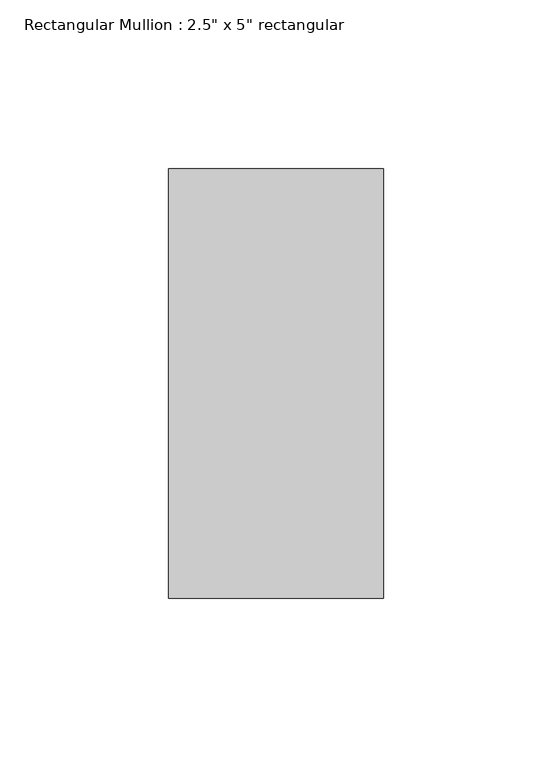
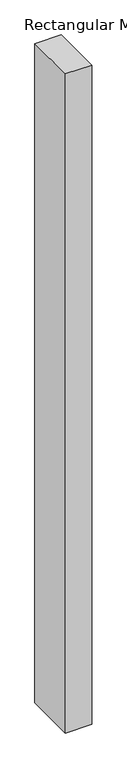
"""IFC4 building model written with IfcOpenShell, lengths in millimetres: member geometry."""

from ifc_helpers import new_model, si_unit, frame, origin, place, context, project, spatial, polyline, outline, extrude, source, transform, mapped, element, save


def member_1f83c645(model_context):
    return source(origin(), model_context, "Body", "SweptSolid", [
        extrude(outline(polyline([(31.75, 63.5), (31.75, -63.5), (-31.75, -63.5), (-31.75, 63.5), (31.75, 63.5)])), frame((0.0, 0.0, -1677.4900448), z_axis=(0.0, 0.0, 1.0), x_axis=(1.0, 0.0, 0.0)), (0.0, 0.0, 1.0), 1677.4900448),
    ])


if __name__ == "__main__":
    model = new_model("IFC4")
    model_context = context("Model", 3, world=origin())
    ifc_project = project(units=[si_unit("LENGTHUNIT", "METRE", prefix="MILLI")], contexts=[model_context])
    site = spatial("IfcSite", under=ifc_project)
    building = spatial("IfcBuilding", under=site)
    placement = place(None, origin())
    member_shape = member_1f83c645(model_context)
    element("IfcMember", 1, ObjectType="Rectangular Mullion : 2.5\" x 5\" rectangular", at=placement, inside=building, context=model_context, shape_type="MappedRepresentation", body=[
        mapped(member_shape, transform((0.0, 0.0, 0.0), x_axis=(1.0, 0.0, 0.0), y_axis=(0.0, 1.0, 0.0), z_axis=(0.0, 0.0, 1.0))),
    ])
    save(model, "model.ifc")

# Revit data of these elements
# Type "Rectangular Mullion : 2.5\" x 5\" rectangular"
#   built-in parameter 1007304 = 0.416667 (stored number, unit not read)
#   built-in parameter 1007301 = 0.104167 (stored number, unit not read)
#   built-in parameter 1007300 = 0.104167 (stored number, unit not read)
# Element 1 (IfcMember, "Rectangular Mullion : 2.5\" x 5\" rectangular")
#   Materials on its faces: "Aluminum"
# Materials
#   "Aluminum": class "Metal", colour RGB 247 247 247, transparency 0, Description = "Aluminum 6061", Cost = 0
